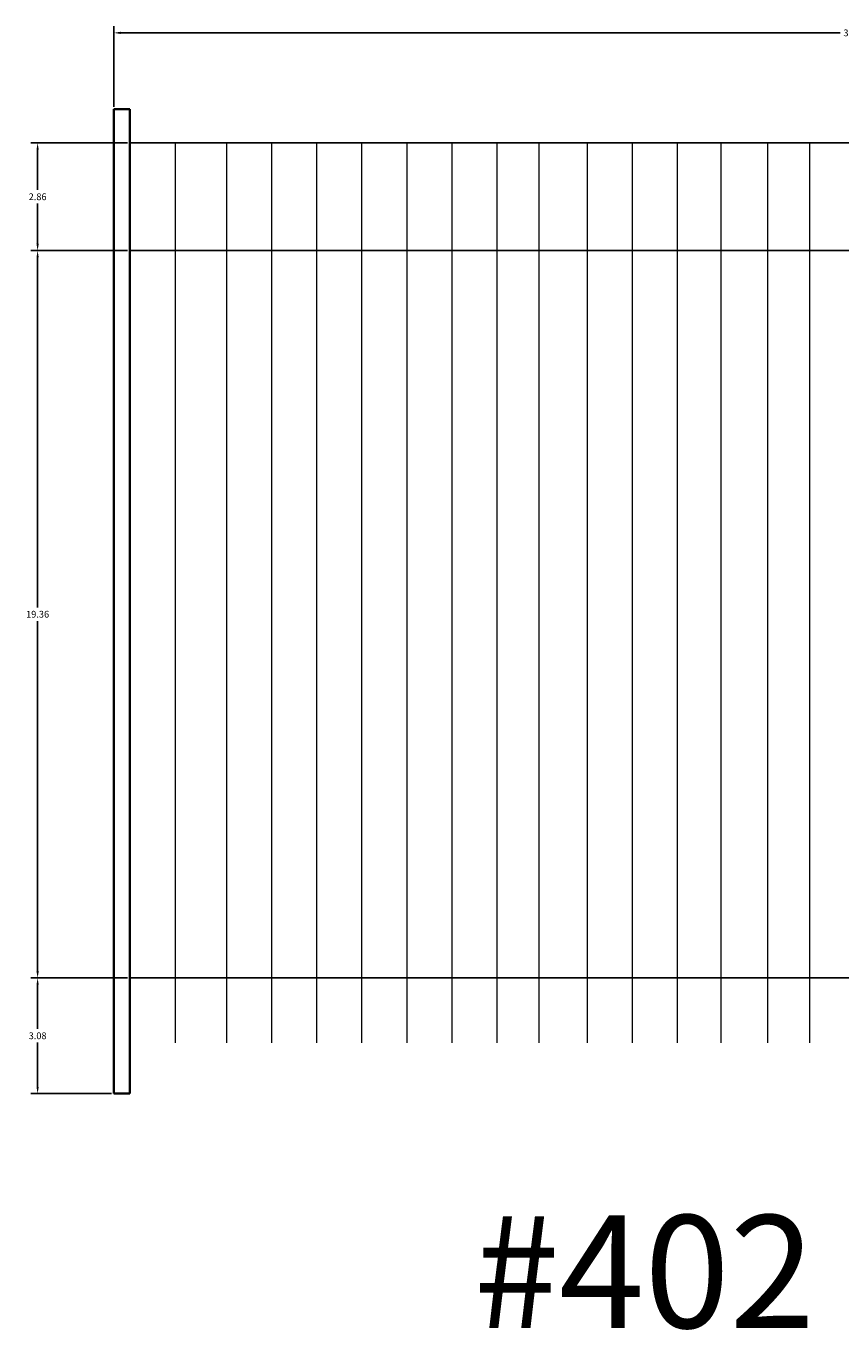
# Model space of a CAD drawing. Units: inches. Extents: x 756 to 915, y 488 to 695.
# Tile 21 of 25: x 864 to 885, y 588 to 622. Entities that reach past the tile are written whole.
import ezdxf

# ---------------------------------------------------------------- set-up
doc = ezdxf.new("R2010")
doc.units = ezdxf.units.IN
doc.header["$MEASUREMENT"] = 0
for name, color, linetype, lineweight in [('L-ANNO-TEXT', 7, 'Continuous', 25), ('L-FENC-PCKT', 7, 'Continuous', 18), ('L-FENC-POST', 7, 'Continuous', 35), ('L-FENC-RAIL', 7, 'Continuous', 25), ('M-DIMS', 2, 'Continuous', 18)]:
    doc.layers.add(name, color=color, linetype=linetype, lineweight=lineweight)
doc.styles.get("Standard").update_dxf_attribs({"font": 'arial.ttf'})
doc.dimstyles.get("Standard").update_dxf_attribs({"dimtxt": 0.18, "dimasz": 0.18, "dimexe": 0.18, "dimexo": 0.0625, "dimgap": 0.09, "dimtad": 0, "dimtih": 1, "dimtoh": 1, "dimdec": 0, "dimzin": 0, "dimdsep": 46, "dimlunit": 3, "dimtxsty": 'Standard', "dimcen": 0.09, "dimadec": 0, "dimazin": 0, "dimtfac": 1, "dimtdec": 0, "dimtofl": 0, "dimtmove": 0, "dimatfit": 3, "dimfxl": 1, "dimtolj": 1, "dimtzin": 0, "dimarcsym": 0})

# ---------------------------------------------------------------- blocks, each defined once
blk = doc.blocks.new('FENCE-POST-LEFT')
for p, q in [((0, 26.207), (0, 0)), ((0, 26.207), (0.426, 26.207)), ((0.426, 26.207), (0.426, 0)), ((0.426, 26.207), (0.426, 0)), ((0, 0), (0.426, 0))]:
    blk.add_line(p, q)
blk = doc.blocks.new('*D44')
at = {"layer": 'Defpoints', "color": 0, "transparency": 16777216}
for p in [(905.412, 622.071), (865.954, 620.041), (905.412, 620.041)]:
    blk.add_point(p, dxfattribs=at)
at = {"layer": 'M-DIMS', "color": 0, "lineweight": -2, "transparency": 16777216}
for p, q in [((865.954, 620.104), (865.954, 622.251)), ((866.134, 622.071), (885.289, 622.071)), ((905.232, 622.071), (886.076, 622.071)), ((905.412, 620.104), (905.412, 622.251))]:
    blk.add_line(p, q, dxfattribs=at)
at = {"layer": 'M-DIMS', "color": 0, "transparency": 16777216}
for points in [[(866.134, 622.101), (866.134, 622.041), (865.954, 622.071)], [(905.232, 622.101), (905.232, 622.041), (905.412, 622.071)]]:
    blk.add_solid(points, dxfattribs=at)
at = {"layer": 'M-DIMS', "color": 0, "transparency": 16777216, "insert": (885.683, 622.071), "char_height": 0.18, "attachment_point": 5}
blk.add_mtext('\\A1;39.46', dxfattribs=at)
blk = doc.blocks.new('*D46')
at = {"layer": 'Defpoints', "color": 0, "transparency": 16777216}
for p in [(863.924, 596.916), (866.38, 596.916), (865.954, 593.835)]:
    blk.add_point(p, dxfattribs=at)
at = {"layer": 'M-DIMS', "color": 0, "lineweight": -2, "transparency": 16777216}
for p, q in [((866.318, 596.916), (863.744, 596.916)), ((863.924, 596.736), (863.924, 595.557)), ((863.924, 594.015), (863.924, 595.194)), ((865.891, 593.835), (863.744, 593.835))]:
    blk.add_line(p, q, dxfattribs=at)
at = {"layer": 'M-DIMS', "color": 0, "transparency": 16777216}
for points in [[(863.894, 596.736), (863.954, 596.736), (863.924, 596.916)], [(863.894, 594.015), (863.954, 594.015), (863.924, 593.835)]]:
    blk.add_solid(points, dxfattribs=at)
at = {"layer": 'M-DIMS', "color": 0, "transparency": 16777216, "insert": (863.924, 595.375), "char_height": 0.18, "attachment_point": 5}
blk.add_mtext('\\A1;3.08', dxfattribs=at)
blk = doc.blocks.new('*D47')
at = {"layer": 'Defpoints', "color": 0, "transparency": 16777216}
for p in [(863.924, 616.276), (866.38, 616.276), (866.38, 596.916)]:
    blk.add_point(p, dxfattribs=at)
at = {"layer": 'M-DIMS', "color": 0, "lineweight": -2, "transparency": 16777216}
for p, q in [((866.318, 616.276), (863.744, 616.276)), ((863.924, 616.096), (863.924, 606.778)), ((863.924, 597.096), (863.924, 606.414)), ((866.318, 596.916), (863.744, 596.916))]:
    blk.add_line(p, q, dxfattribs=at)
at = {"layer": 'M-DIMS', "color": 0, "transparency": 16777216}
for points in [[(863.894, 616.096), (863.954, 616.096), (863.924, 616.276)], [(863.894, 597.096), (863.954, 597.096), (863.924, 596.916)]]:
    blk.add_solid(points, dxfattribs=at)
at = {"layer": 'M-DIMS', "color": 0, "transparency": 16777216, "insert": (863.924, 606.596), "char_height": 0.18, "attachment_point": 5}
blk.add_mtext('\\A1;19.36', dxfattribs=at)
blk = doc.blocks.new('*D48')
at = {"layer": 'Defpoints', "color": 0, "transparency": 16777216}
for p in [(863.924, 619.14), (866.38, 619.14), (866.38, 616.276)]:
    blk.add_point(p, dxfattribs=at)
at = {"layer": 'M-DIMS', "color": 0, "lineweight": -2, "transparency": 16777216}
for p, q in [((866.318, 619.14), (863.744, 619.14)), ((863.924, 618.96), (863.924, 617.89)), ((863.924, 616.456), (863.924, 617.526)), ((866.318, 616.276), (863.744, 616.276))]:
    blk.add_line(p, q, dxfattribs=at)
at = {"layer": 'M-DIMS', "color": 0, "transparency": 16777216}
for points in [[(863.894, 618.96), (863.954, 618.96), (863.924, 619.14)], [(863.894, 616.456), (863.954, 616.456), (863.924, 616.276)]]:
    blk.add_solid(points, dxfattribs=at)
at = {"layer": 'M-DIMS', "color": 0, "transparency": 16777216, "insert": (863.924, 617.708), "char_height": 0.18, "attachment_point": 5}
blk.add_mtext('\\A1;2.86', dxfattribs=at)

msp = doc.modelspace()

# ---------------------------------------------------------------- linework, layer by layer
at = {"layer": 'L-FENC-PCKT'}
for p, q in [((867.5865, 619.1305), (867.5865, 595.1842)), ((868.9528, 619.1305), (868.9528, 595.1842)), ((870.1478, 619.1305), (870.1478, 595.1842)), ((871.3527, 619.1305), (871.3527, 595.1842)), ((872.549, 619.1305), (872.549, 595.1842)), ((873.7526, 619.1305), (873.7526, 595.1842)), ((874.9502, 619.1305), (874.9502, 595.1842)), ((876.1525, 619.1305), (876.1525, 595.1842)), ((877.2714, 619.1305), (877.2714, 595.1842)), ((878.5524, 619.1305), (878.5524, 595.1842)), ((879.7527, 619.1305), (879.7527, 595.1842)), ((880.9523, 619.1305), (880.9523, 595.1842)), ((882.1139, 619.1305), (882.1139, 595.1842)), ((883.3522, 619.1305), (883.3522, 595.1842)), ((884.4751, 619.1305), (884.4751, 595.1842))]:
    msp.add_line(p, q, dxfattribs=at)
at = {"layer": 'L-FENC-RAIL'}
for p, q in [((866.3803, 619.1401), (904.9851, 619.1401)), ((866.3803, 616.2757), (904.9851, 616.2757)), ((866.3803, 596.9163), (904.9851, 596.9163))]:
    msp.add_line(p, q, dxfattribs=at)

# ---------------------------------------------------------------- block references
at = {"layer": 'L-FENC-POST'}
msp.add_blockref('FENCE-POST-LEFT', (865.954, 593.8346), dxfattribs=at)

# ---------------------------------------------------------------- texts
at = {"layer": 'L-ANNO-TEXT'}
msp.add_text('#402', height=3, dxfattribs=at).set_placement((875.535, 587.5988))

# ---------------------------------------------------------------- dimensions: what is measured, and where the dimension line sits
at = {"layer": 'M-DIMS'}
dim = msp.add_linear_dim(base=(905.4118, 622.0715), p1=(865.9536, 620.0415), p2=(905.4118, 620.0415), dimstyle='Standard', override={"dimdec": 2, "dimlfac": 1, "dimrnd": 0, "dimzin": 0, "dimdsep": 46, "dimlunit": 2}, dxfattribs=at)
dim.commit()
dim.dimension.update_dxf_attribs({"geometry": '*D44', "text_midpoint": (885.6827, 622.0715)})
for base, p1, p2, picture, middle in [((863.9236, 619.1401), (866.3803, 616.2757), (866.3803, 619.1401), '*D48', (863.9236, 617.7079)), ((863.9236, 616.2757), (866.3803, 596.9163), (866.3803, 616.2757), '*D47', (863.9236, 606.596)), ((863.9236, 596.9163), (865.9536, 593.8347), (866.3803, 596.9163), '*D46', (863.9236, 595.3755))]:
    dim = msp.add_linear_dim(base=base, p1=p1, p2=p2, angle=90, dimstyle='Standard', override={"dimdec": 2, "dimlfac": 1, "dimrnd": 0, "dimzin": 0, "dimdsep": 46, "dimlunit": 2}, dxfattribs=at)
    dim.commit()
    dim.dimension.update_dxf_attribs({"geometry": picture, "text_midpoint": middle})

doc.saveas('drawing.dxf')
